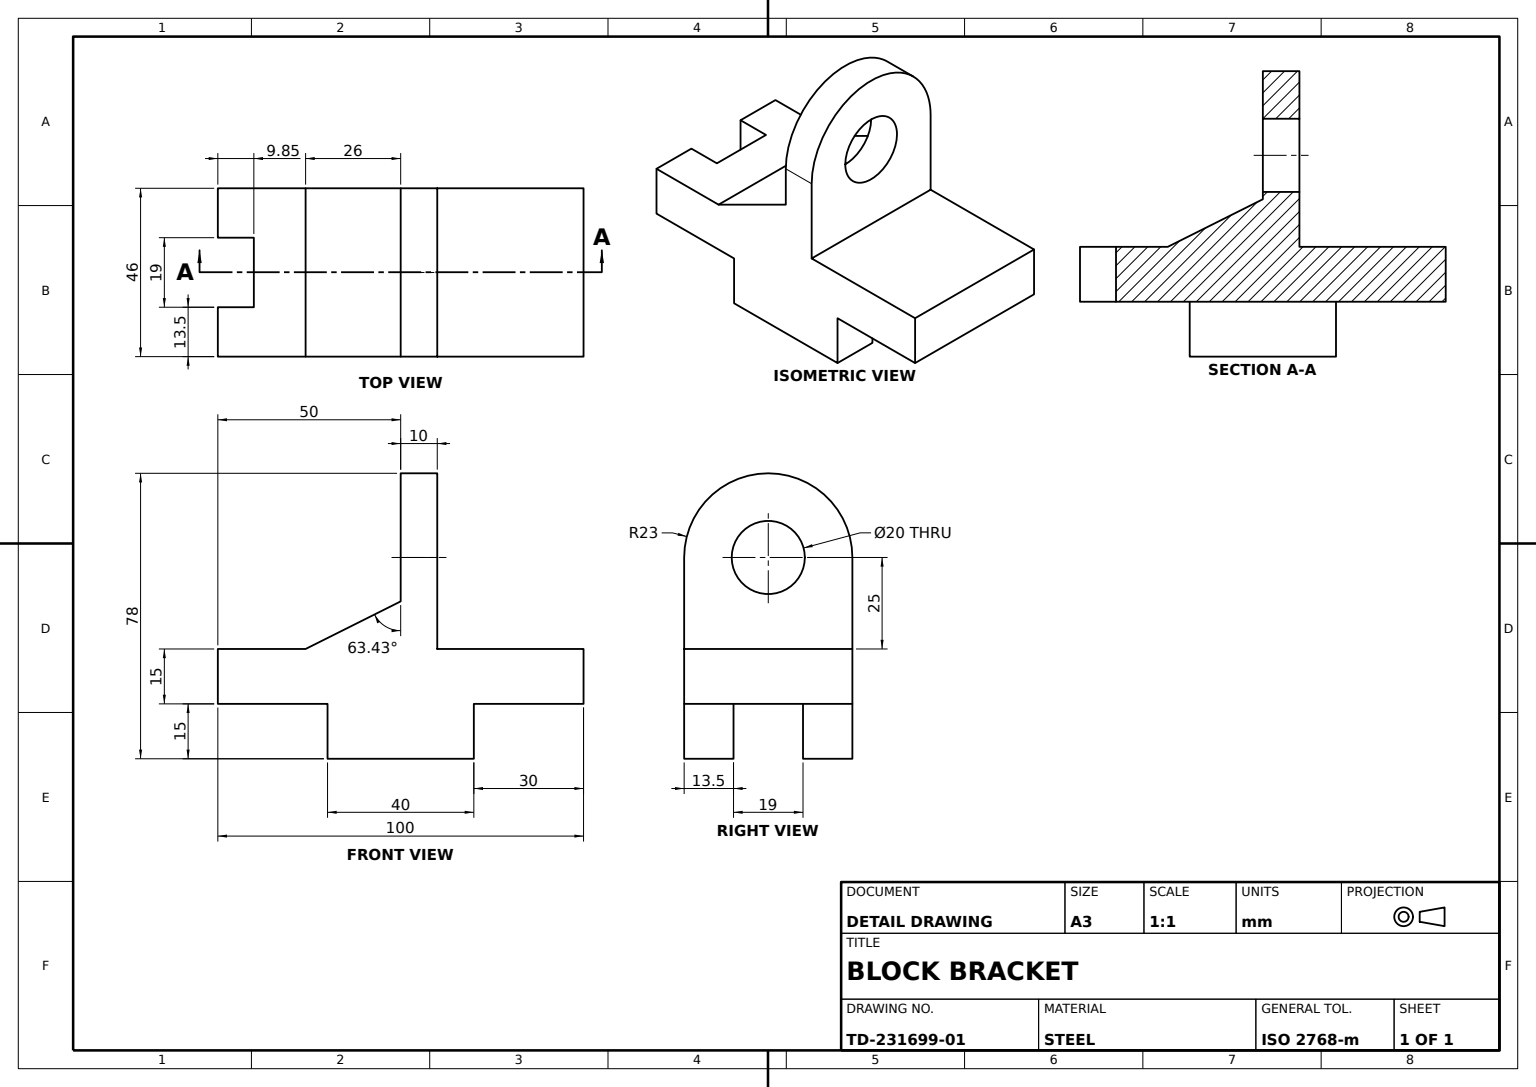
from build123d import *
from build123d.topology import SkipClean

# Parameters (mm, degrees)
BASE_PLATE_DEPTH      = 15
SIDE_BLOCK_A_SKETCH_W = 40
SIDE_BLOCK_A_SKETCH_H = 15
SIDE_BLOCK_A_DEPTH    = 13.5
SIDE_BLOCK_B_SKETCH_W = 40
SIDE_BLOCK_B_SKETCH_H = 15
SIDE_BLOCK_B_DEPTH    = 13.5
UPRIGHT_WEB_SKETCH_W  = 46
UPRIGHT_WEB_SKETCH_H  = 10
UPRIGHT_WEB_DEPTH     = 25
LUG_EAR_DEPTH         = 10
LUG_HOLE_SKETCH_R     = 10
LUG_HOLE_DEPTH        = 10
GUSSET_DEPTH          = 46


with BuildPart() as part:
    # Base Plate Sketch → Base Plate (new body)
    with BuildSketch(Plane(origin=(0, 0, 0), x_dir=(1, 0, 0), z_dir=(0, 1, 0))):
        Polygon((13.5, 0), (13.5, 9.84759163), (32.5, 9.84759163), (32.5, 0), (46, 0), (46, 100), (0, 100), (0, 0), align=None)
    extrude(amount=BASE_PLATE_DEPTH)

    # Side Block A Sketch → Side Block A (add)
    with BuildSketch(Plane(origin=(0, 0, 0), x_dir=(0, 0, -1), z_dir=(1, 0, 0))):
        with Locations((50, -7.5)):
            Rectangle(SIDE_BLOCK_A_SKETCH_W, SIDE_BLOCK_A_SKETCH_H)
    extrude(amount=SIDE_BLOCK_A_DEPTH)

    # Side Block B Sketch → Side Block B (add)
    with BuildSketch(Plane(origin=(46, 0, 0), x_dir=(0, 0, -1), z_dir=(1, 0, 0))):
        with Locations((50, -7.5)):
            Rectangle(SIDE_BLOCK_B_SKETCH_W, SIDE_BLOCK_B_SKETCH_H)
    extrude(amount=-SIDE_BLOCK_B_DEPTH)

    # Upright Web Sketch → Upright Web (add)
    with BuildSketch(Plane(origin=(0, 15, 0), x_dir=(1, 0, 0), z_dir=(0, 1, 0))):
        with Locations((23, 55)):
            Rectangle(UPRIGHT_WEB_SKETCH_W, UPRIGHT_WEB_SKETCH_H)
    extrude(amount=UPRIGHT_WEB_DEPTH)

    # Lug Ear Sketch → Lug Ear (add)
    with BuildSketch(Plane.XY.offset(-50)):
        with BuildLine():
            ThreePointArc((33, 40), (23, 30), (13, 40))
            Line((13, 40), (0, 40))
            ThreePointArc((0, 40), (23, 17), (46, 40))
            Line((46, 40), (33, 40))
        make_face()
        with BuildLine():
            Line((0, 40), (13, 40))
            ThreePointArc((13, 40), (23, 50), (33, 40))
            Line((33, 40), (46, 40))
            ThreePointArc((46, 40), (23, 63), (0, 40))
        make_face()
    extrude(amount=-LUG_EAR_DEPTH)

    # Lug Hole Sketch → Lug Hole (cut)
    with SkipClean():  # the faces are left unmerged after this step: merging them gives an invalid solid
        with BuildSketch(Plane.XY.offset(-50)):
            with Locations((23, 40)):
                Circle(LUG_HOLE_SKETCH_R)
        extrude(amount=-LUG_HOLE_DEPTH, mode=Mode.SUBTRACT)

    # Gusset Sketch → Gusset (add)
    with SkipClean():  # the faces are left unmerged after this step: merging them gives an invalid solid
        with BuildSketch(Plane(origin=(46, 0, 0), x_dir=(0, 0, -1), z_dir=(1, 0, 0))):
            Polygon((50, 15), (24, 15), (50, 28), align=None)
        extrude(amount=-GUSSET_DEPTH)


solid = part.part
